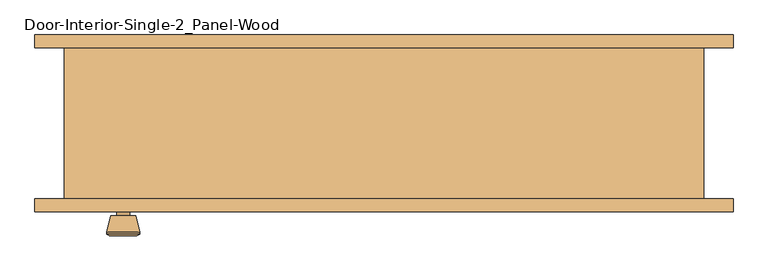
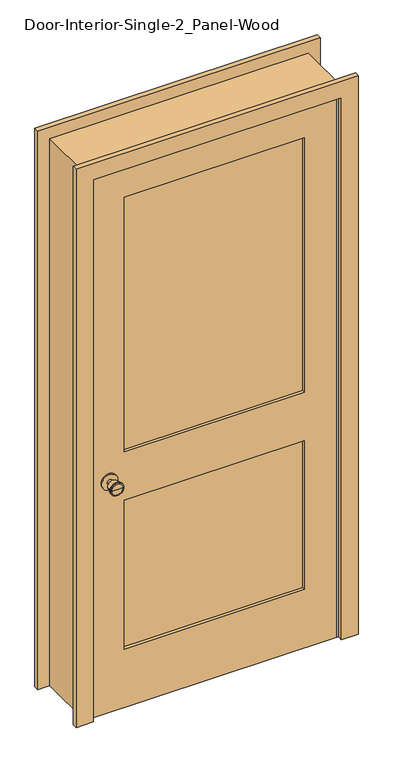
"""IFC4 building model written with IfcOpenShell, lengths in millimetres: door geometry, Door-Interior-Single-2_Panel-Wood."""

from ifc_helpers import new_model, si_unit, point, frame, frame_2d, origin, place, context, project, spatial, polyline, circle_curve, trimmed, segment, composite_curve, outline, extrude, faceted_brep, source, transform, mapped, element, save
from ifc_brep_helpers import plane_surface, cylinder_surface, revolved_surface, advanced_brep


def door_interior_single_2_panel_wood_5dd36918(model_context):
    return source(origin(), model_context, "Body", "SolidModel", [
        advanced_brep(
        [(-393.7, -70.2, 914.4), (-403.7, -70.2, 914.4), (-383.7, -70.2, 914.4), (-373.2241324, -21.2, 914.4), (-414.1758676, -21.2, 914.4), (-393.7, -21.2, 914.4), (-368.7, -23.0278681, 914.4), (-418.7, -23.0278681, 914.4), (-368.7, -26.4915463, 914.4), (-418.7, -26.4915463, 914.4), (-375.063764, -51.2, 914.4), (-412.336236, -51.2, 914.4), (-383.7, -51.2, 914.4), (-403.7, -51.2, 914.4)],
        [
            (0, 1),
            (1, 2, circle_curve(frame((-393.7, -70.2, 914.4), z_axis=(0.0, -1.0, 0.0), x_axis=(-1.0, 0.0, 0.0)), 10.0)),
            (2, 0),
            (2, 1, circle_curve(frame((-393.7, -70.2, 914.4), z_axis=(0.0, -1.0, 0.0), x_axis=(-1.0, 0.0, 0.0)), 10.0)),
            (3, 4, circle_curve(frame((-393.7, -21.2, 914.4), z_axis=(0.0, 1.0, 0.0), x_axis=(-1.0, 0.0, 0.0)), 20.4758676)),
            (4, 5),
            (5, 3),
            (4, 3, circle_curve(frame((-393.7, -21.2, 914.4), z_axis=(0.0, 1.0, 0.0), x_axis=(-1.0, 0.0, 0.0)), 20.4758676)),
            (6, 7, circle_curve(frame((-393.7, -23.0278681, 914.4), z_axis=(0.0, 1.0, 0.0), x_axis=(-1.0, 0.0, 0.0)), 25.0)),
            (7, 4),
            (3, 6),
            (7, 6, circle_curve(frame((-393.7, -23.0278681, 914.4), z_axis=(0.0, 1.0, 0.0), x_axis=(-1.0, 0.0, 0.0)), 25.0)),
            (8, 9, circle_curve(frame((-393.7, -26.4915463, 914.4), z_axis=(0.0, 1.0, 0.0), x_axis=(-1.0, 0.0, 0.0)), 25.0)),
            (9, 7),
            (6, 8),
            (9, 8, circle_curve(frame((-393.7, -26.4915463, 914.4), z_axis=(0.0, 1.0, 0.0), x_axis=(-1.0, 0.0, 0.0)), 25.0)),
            (10, 11, circle_curve(frame((-393.7, -51.2, 914.4), z_axis=(0.0, 1.0, 0.0), x_axis=(-1.0, 0.0, 0.0)), 18.636236)),
            (11, 9),
            (8, 10),
            (11, 10, circle_curve(frame((-393.7, -51.2, 914.4), z_axis=(0.0, 1.0, 0.0), x_axis=(-1.0, 0.0, 0.0)), 18.636236)),
            (12, 13, circle_curve(frame((-393.7, -51.2, 914.4), z_axis=(0.0, 1.0, 0.0), x_axis=(-1.0, 0.0, 0.0)), 10.0)),
            (13, 11),
            (10, 12),
            (13, 12, circle_curve(frame((-393.7, -51.2, 914.4), z_axis=(0.0, 1.0, 0.0), x_axis=(-1.0, 0.0, 0.0)), 10.0)),
            (1, 13),
            (12, 2),
        ],
        [
            plane_surface(frame((-393.7, -70.2, 914.4), z_axis=(0.0, -1.0, 0.0), x_axis=(-1.0, 0.0, 0.0))),
            plane_surface(frame((-393.7, -21.2, 914.4), z_axis=(0.0, 1.0, 0.0), x_axis=(-1.0, 0.0, 0.0))),
            revolved_surface(polyline([(-414.1758676, -21.2, 914.4), (-418.7, -23.0278681, 914.4)]), (-393.7, -70.2, 914.4), (0.0, -1.0, 0.0)),
            cylinder_surface(frame((-393.7, -70.2, 914.4), z_axis=(0.0, -1.0, 0.0), x_axis=(-1.0, 0.0, 0.0)), 25.0),
            revolved_surface(polyline([(-418.7, -26.4915463, 914.4), (-412.336236, -51.2, 914.4)]), (-393.7, -70.2, 914.4), (0.0, -1.0, 0.0)),
            plane_surface(frame((-393.7, -51.2, 914.4), z_axis=(0.0, -1.0, 0.0), x_axis=(-1.0, 0.0, 0.0))),
            cylinder_surface(frame((-393.7, -70.2, 914.4), z_axis=(0.0, -1.0, 0.0), x_axis=(-1.0, 0.0, 0.0)), 10.0),
        ],
        [
            (0, [[1, 2, 3]]),
            (0, [[-3, 4, -1]]),
            (1, [[5, 6, 7]]),
            (1, [[8, -7, -6]]),
            (2, [[9, 10, -5, 11]]),
            (2, [[12, -11, -8, -10]]),
            (3, [[13, 14, -9, 15]]),
            (3, [[16, -15, -12, -14]]),
            (4, [[17, 18, -13, 19]]),
            (4, [[20, -19, -16, -18]]),
            (5, [[21, 22, -17, 23]]),
            (5, [[24, -23, -20, -22]]),
            (6, [[-2, 25, -21, 26]]),
            (6, [[-4, -26, -24, -25]]),
        ],
    ),
        extrude(outline(composite_curve([segment(trimmed(circle_curve(frame_2d((914.4, -393.7)), 30.0), [point((914.4, -423.7))], [point((914.4, -363.7))], False, "CARTESIAN"), True, "CONTINUOUS"), segment(trimmed(circle_curve(frame_2d((914.4, -393.7)), 30.0), [point((914.4, -363.7))], [point((914.4, -423.7))], False, "CARTESIAN"), True, "CONTINUOUS")], self_intersect=False)), frame((0.0, -76.2, 0.0), z_axis=(0.0, 1.0, 0.0), x_axis=(0.0, 0.0, 1.0)), (0.0, 0.0, 1.0), 6.0),
        advanced_brep(
        [(-393.7, -117.125, 914.4), (-383.7, -117.125, 914.4), (-403.7, -117.125, 914.4), (-373.2241324, -166.125, 914.4), (-393.7, -166.125, 914.4), (-414.1758676, -166.125, 914.4), (-368.7, -164.2971319, 914.4), (-418.7, -164.2971319, 914.4), (-368.7, -160.8334537, 914.4), (-418.7, -160.8334537, 914.4), (-375.063764, -136.125, 914.4), (-412.336236, -136.125, 914.4), (-383.7, -136.125, 914.4), (-403.7, -136.125, 914.4)],
        [
            (0, 1),
            (1, 2, circle_curve(frame((-393.7, -117.125, 914.4), z_axis=(0.0, 1.0, 0.0), x_axis=(-1.0, 0.0, 0.0)), 10.0)),
            (2, 0),
            (2, 1, circle_curve(frame((-393.7, -117.125, 914.4), z_axis=(0.0, 1.0, 0.0), x_axis=(-1.0, 0.0, 0.0)), 10.0)),
            (3, 4),
            (4, 5),
            (5, 3, circle_curve(frame((-393.7, -166.125, 914.4), z_axis=(0.0, -1.0, 0.0), x_axis=(-1.0, 0.0, 0.0)), 20.4758676)),
            (3, 5, circle_curve(frame((-393.7, -166.125, 914.4), z_axis=(0.0, -1.0, 0.0), x_axis=(-1.0, 0.0, 0.0)), 20.4758676)),
            (6, 3),
            (5, 7),
            (7, 6, circle_curve(frame((-393.7, -164.2971319, 914.4), z_axis=(0.0, -1.0, 0.0), x_axis=(-1.0, 0.0, 0.0)), 25.0)),
            (6, 7, circle_curve(frame((-393.7, -164.2971319, 914.4), z_axis=(0.0, -1.0, 0.0), x_axis=(-1.0, 0.0, 0.0)), 25.0)),
            (8, 6),
            (7, 9),
            (9, 8, circle_curve(frame((-393.7, -160.8334537, 914.4), z_axis=(0.0, -1.0, 0.0), x_axis=(-1.0, 0.0, 0.0)), 25.0)),
            (8, 9, circle_curve(frame((-393.7, -160.8334537, 914.4), z_axis=(0.0, -1.0, 0.0), x_axis=(-1.0, 0.0, 0.0)), 25.0)),
            (10, 8),
            (9, 11),
            (11, 10, circle_curve(frame((-393.7, -136.125, 914.4), z_axis=(0.0, -1.0, 0.0), x_axis=(-1.0, 0.0, 0.0)), 18.636236)),
            (10, 11, circle_curve(frame((-393.7, -136.125, 914.4), z_axis=(0.0, -1.0, 0.0), x_axis=(-1.0, 0.0, 0.0)), 18.636236)),
            (12, 10),
            (11, 13),
            (13, 12, circle_curve(frame((-393.7, -136.125, 914.4), z_axis=(0.0, -1.0, 0.0), x_axis=(-1.0, 0.0, 0.0)), 10.0)),
            (12, 13, circle_curve(frame((-393.7, -136.125, 914.4), z_axis=(0.0, -1.0, 0.0), x_axis=(-1.0, 0.0, 0.0)), 10.0)),
            (1, 12),
            (13, 2),
        ],
        [
            plane_surface(frame((-393.7, -117.125, 914.4), z_axis=(0.0, 1.0, 0.0), x_axis=(-1.0, 0.0, 0.0))),
            plane_surface(frame((-393.7, -166.125, 914.4), z_axis=(0.0, -1.0, 0.0), x_axis=(-1.0, 0.0, 0.0))),
            revolved_surface(polyline([(-414.1758676, -166.125, 914.4), (-418.7, -164.2971319, 914.4)]), (-393.7, -117.125, 914.4), (0.0, 1.0, 0.0)),
            cylinder_surface(frame((-393.7, -117.125, 914.4), z_axis=(0.0, 1.0, 0.0), x_axis=(-1.0, 0.0, 0.0)), 25.0),
            revolved_surface(polyline([(-418.7, -160.8334537, 914.4), (-412.336236, -136.125, 914.4)]), (-393.7, -117.125, 914.4), (0.0, 1.0, 0.0)),
            plane_surface(frame((-393.7, -136.125, 914.4), z_axis=(0.0, 1.0, 0.0), x_axis=(-1.0, 0.0, 0.0))),
            cylinder_surface(frame((-393.7, -117.125, 914.4), z_axis=(0.0, 1.0, 0.0), x_axis=(-1.0, 0.0, 0.0)), 10.0),
        ],
        [
            (0, [[1, 2, 3]]),
            (0, [[-3, 4, -1]]),
            (1, [[5, 6, 7]]),
            (1, [[-6, -5, 8]]),
            (2, [[9, -7, 10, 11]]),
            (2, [[-10, -8, -9, 12]]),
            (3, [[13, -11, 14, 15]]),
            (3, [[-14, -12, -13, 16]]),
            (4, [[17, -15, 18, 19]]),
            (4, [[-18, -16, -17, 20]]),
            (5, [[21, -19, 22, 23]]),
            (5, [[-22, -20, -21, 24]]),
            (6, [[25, -23, 26, -2]]),
            (6, [[-26, -24, -25, -4]]),
        ],
    ),
        extrude(outline(composite_curve([segment(trimmed(circle_curve(frame_2d((914.4, -393.7)), 30.0), [point((914.4, -423.7))], [point((914.4, -363.7))], False, "CARTESIAN"), True, "CONTINUOUS"), segment(trimmed(circle_curve(frame_2d((914.4, -393.7)), 30.0), [point((914.4, -363.7))], [point((914.4, -423.7))], False, "CARTESIAN"), True, "CONTINUOUS")], self_intersect=False)), frame((0.0, -117.125, 0.0), z_axis=(0.0, 1.0, 0.0), x_axis=(0.0, 0.0, 1.0)), (0.0, 0.0, 1.0), 6.0),
        faceted_brep([(482.6, -111.125, 0.0), (457.2, -111.125, 0.0), (457.2, -76.2, 0.0), (444.5, -76.2, 0.0), (444.5, -41.275, 0.0), (457.2, -41.275, 0.0), (457.2, 117.475, 0.0), (482.6, 117.475, 0.0), (482.6, 117.475, 2159.0), (482.6, -111.125, 2159.0), (457.2, 117.475, 2133.6), (-457.2, 117.475, 2133.6), (-457.2, 117.475, 0.0), (-482.6, 117.475, 0.0), (-482.6, 117.475, 2159.0), (457.2, -41.275, 2133.6), (444.5, -41.275, 2120.9), (-444.5, -41.275, 2120.9), (-444.5, -41.275, 0.0), (-457.2, -41.275, 0.0), (-457.2, -41.275, 2133.6), (444.5, -76.2, 2120.9), (457.2, -76.2, 2133.6), (-457.2, -76.2, 2133.6), (-457.2, -76.2, 0.0), (-444.5, -76.2, 0.0), (-444.5, -76.2, 2120.9), (457.2, -111.125, 2133.6), (-482.6, -111.125, 2159.0), (-482.6, -111.125, 0.0), (-457.2, -111.125, 0.0), (-457.2, -111.125, 2133.6)], [[[0, 1, 2, 3, 4, 5, 6, 7]], [[7, 8, 9, 0]], [[6, 10, 11, 12, 13, 14, 8, 7]], [[5, 15, 10, 6]], [[4, 16, 17, 18, 19, 20, 15, 5]], [[3, 21, 16, 4]], [[2, 22, 23, 24, 25, 26, 21, 3]], [[1, 27, 22, 2]], [[0, 9, 28, 29, 30, 31, 27, 1]], [[8, 14, 28, 9]], [[15, 20, 11, 10]], [[21, 26, 17, 16]], [[27, 31, 23, 22]], [[29, 13, 12, 19, 18, 25, 24, 30]], [[14, 13, 29, 28]], [[20, 19, 12, 11]], [[26, 25, 18, 17]], [[31, 30, 24, 23]]]),
        extrude(outline(polyline([(2133.6, -457.2), (0.0, -457.2), (0.0, 457.2), (2133.6, 457.2), (2133.6, -457.2)]), holes=[polyline([(2014.5375, -336.55), (2014.5375, 336.55), (1009.65, 336.55), (1009.65, -336.55), (2014.5375, -336.55)]), polyline([(819.15, -336.55), (819.15, 336.55), (231.775, 336.55), (231.775, -336.55), (819.15, -336.55)])]), frame((0.0, -111.125, 0.0), z_axis=(0.0, 1.0, 0.0), x_axis=(0.0, 0.0, 1.0)), (0.0, 0.0, 1.0), 34.925),
        extrude(outline(polyline([(336.55, -87.8416667), (336.55, -99.4833333), (-336.55, -99.4833333), (-336.55, -87.8416667), (336.55, -87.8416667)])), frame((0.0, 0.0, 1009.65), z_axis=(0.0, 0.0, 1.0), x_axis=(1.0, 0.0, 0.0)), (0.0, 0.0, 1.0), 1004.8875),
        extrude(outline(polyline([(336.55, -87.8416667), (336.55, -99.4833333), (-336.55, -99.4833333), (-336.55, -87.8416667), (336.55, -87.8416667)])), frame((0.0, 0.0, 231.775), z_axis=(0.0, 0.0, 1.0), x_axis=(1.0, 0.0, 0.0)), (0.0, 0.0, 1.0), 587.375),
        extrude(outline(polyline([(0.0, 527.05), (2203.45, 527.05), (2203.45, -527.05), (0.0, -527.05), (0.0, -463.55), (2139.95, -463.55), (2139.95, 463.55), (0.0, 463.55), (0.0, 527.05)])), frame((0.0, -130.175, 0.0), z_axis=(0.0, 1.0, 0.0), x_axis=(0.0, 0.0, 1.0)), (0.0, 0.0, 1.0), 19.05),
        extrude(outline(polyline([(0.0, 527.05), (2203.45, 527.05), (2203.45, -527.05), (0.0, -527.05), (0.0, -463.55), (2139.95, -463.55), (2139.95, 463.55), (0.0, 463.55), (0.0, 527.05)])), frame((0.0, 117.475, 0.0), z_axis=(0.0, 1.0, 0.0), x_axis=(0.0, 0.0, 1.0)), (0.0, 0.0, 1.0), 19.05),
    ])


if __name__ == "__main__":
    model = new_model("IFC4")
    model_context = context("Model", 3, world=origin())
    ifc_project = project(units=[si_unit("LENGTHUNIT", "METRE", prefix="MILLI")], contexts=[model_context])
    site = spatial("IfcSite", under=ifc_project)
    building = spatial("IfcBuilding", under=site)
    placement = place(None, origin())
    door_interior_single_2_panel_wood_shape = door_interior_single_2_panel_wood_5dd36918(model_context)
    element("IfcDoor", 1, ObjectType="Door-Interior-Single-2_Panel-Wood", at=placement, inside=building, context=model_context, shape_type="MappedRepresentation", body=[
        mapped(door_interior_single_2_panel_wood_shape, transform((0.0, 0.0, 0.0), x_axis=(1.0, 0.0, 0.0), y_axis=(0.0, 1.0, 0.0), z_axis=(0.0, 0.0, 1.0))),
    ])
    save(model, "model.ifc")

# Revit data of these elements
# Type "Door-Interior-Single-2_Panel-Wood"
#   Type Mark = "10"
#   Assembly Code = "C1020300"
#   Analytic Construction = "Wooden"
#   Top Rail = 0' - 4 11/16"
#   Thickness = 0' - 1 3/8"
#   Thermal Resistance (R) = 2.5876 (h·ft²·°F)/BTU
#   Swing Angle [instance default] = 90.00°
#   Stiles = 0' - 4 3/4"
#   Rough Width = 3' - 2"
#   Rough Height = 7' - 1"
#   Lock Rail = 0' - 7 1/2"
#   Height = 7' - 0"
#   Width = 3' - 0"
#   Heat Transfer Coefficient (U) = 0.3865 BTU/(h·ft²·°F)
#   Bottom Rail = 0' - 9 1/8"
#   Trim Material = Cherry
#   Panel Material = Cherry
#   Frame Material = Cherry
#   Door Handle Material = Aluminum
#   Visual Light Transmittance = 0
#   Solar Heat Gain Coefficient = 0
#   Wall Closure = (empty or 0)
#   Function = (empty or 0)
# Element 1 (IfcDoor, "Door-Interior-Single-2_Panel-Wood")
#   Materials on its faces: "Cherry", "Aluminum"
# Materials
#   "Cherry": class "Wood", colour RGB 226 177 128, transparency 0, Description = "Prunus Serotina", Cost = 0
#   "Aluminum": class "Metal", colour RGB 247 247 247, transparency 0, Description = "Aluminum 6061", Cost = 0
